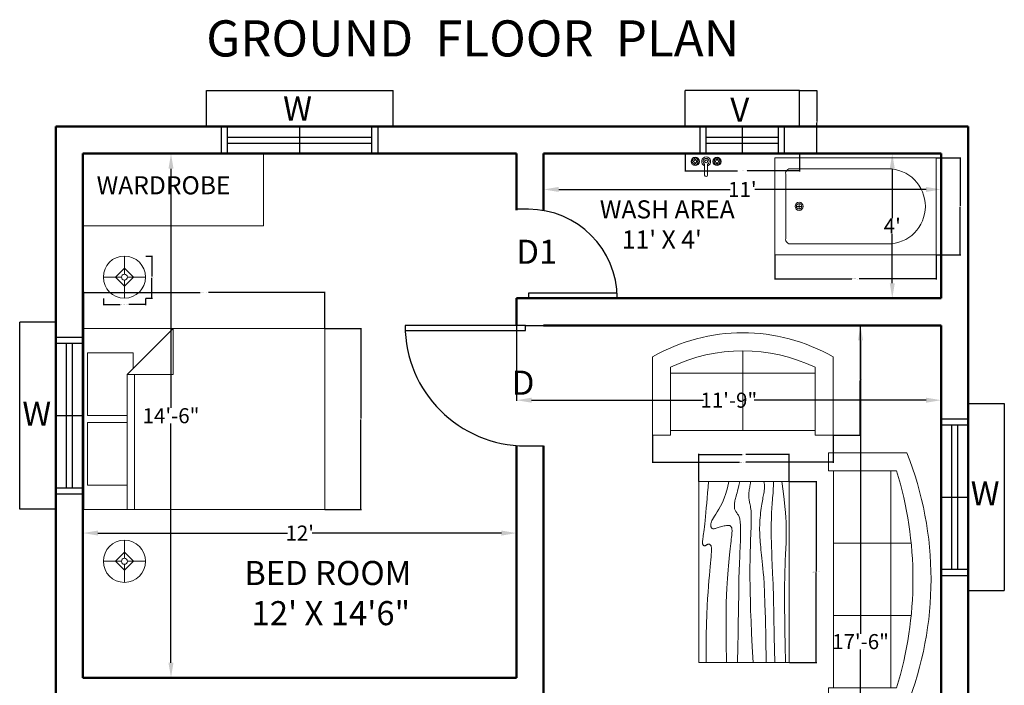
# Model space of a CAD drawing. Units: inches. Extents: x -25 to 789, y -921 to 230.
# Tile 3 of 5: x 5 to 332, y -11 to 209. Entities that reach past the tile are written whole.
import ezdxf

# ---------------------------------------------------------------- set-up
doc = ezdxf.new("R2010")
doc.units = ezdxf.units.IN
doc.header["$MEASUREMENT"] = 0
for name, color, linetype, lineweight in [('A-ANNO-DIMS', 2, 'Continuous', 18), ('A-ANNO-TEXT', 7, 'Continuous', 18), ('A-AREA-IDEN', 3, 'Continuous', 18), ('A-DOOR', 4, 'Continuous', 25), ('A-FLOR-FIXT', 9, 'Continuous', 18), ('A-FURN', 8, 'Continuous', 18), ('A-GLAZ', 4, 'Continuous', 25), ('A-WALL', 7, 'Continuous', 50), ('E-LITE-FIXT', 6, 'Continuous', 18)]:
    doc.layers.add(name, color=color, linetype=linetype, lineweight=lineweight)
doc.styles.get("Standard").update_dxf_attribs({"font": 'arial.ttf'})
doc.dimstyles.get("Standard").update_dxf_attribs({"dimtxt": 0.18, "dimasz": 0.18, "dimexe": 0.18, "dimexo": 0.0625, "dimgap": 0.09, "dimtad": 0, "dimtih": 1, "dimtoh": 1, "dimdec": 1, "dimzin": 0, "dimdsep": 46, "dimlunit": 4, "dimtxsty": 'Standard', "dimcen": 0.09, "dimadec": 0, "dimazin": 0, "dimtfac": 1, "dimtdec": 1, "dimtofl": 0, "dimtmove": 0, "dimatfit": 3, "dimfxl": 1, "dimtolj": 1, "dimtzin": 0, "dimarcsym": 0})

# ---------------------------------------------------------------- blocks, each defined once
blk = doc.blocks.new('*U2')
for p, q in [((0, 0), (0, -6)), ((-40, 0), (-40, -6))]:
    blk.add_line(p, q)
blk.add_lwpolyline([(0, 0), (0, 40), (-1.75, 40), (-1.75, 0)], close=True)
blk.add_arc((0, 0), 40, 90, 180)
blk = doc.blocks.new('*U4')
for p, q in [((-750, 0), (-750, -100)), ((0, 0), (0, -100))]:
    blk.add_line(p, q)
blk.add_lwpolyline([(0, 0), (0, 750), (-43.75, 750), (-43.75, 0)], close=True)
blk.add_arc((0, 0), 750, 90, 180)
blk = doc.blocks.new('Bed - Queen')
for p, q in [((0, -80.00003), (0, 0)), ((0, 0), (59.99999, 0)), ((59.99999, 0), (59.99999, -80.00003)), ((7.99999, -1.2), (28.79998, -1.2)), ((7.99999, -14.4), (7.99999, -1.2)), ((28.79998, -1.2), (28.79998, -14.4)), ((31.19999, -1.2), (51.99999, -1.2)), ((31.19999, -14.4), (31.19999, -1.2)), ((51.99999, -1.2), (51.99999, -16.4)), ((0, -14.4), (44.8, -14.4)), ((59.99999, -29.6), (44.8, -14.4)), ((44.8, -14.4), (44.8, -29.6)), ((44.8, -16.8), (0, -16.8)), ((51.99999, -16.4), (46.79936, -16.4)), ((44.8, -29.6), (59.99999, -29.6)), ((59.99999, -80.00003), (0, -80.00003))]:
    blk.add_line(p, q)
blk = doc.blocks.new('Lamp - Table')
for p, q in [((0, 7), (0, 1)), ((-1, 0), (-7, 0)), ((0, 3), (-3, 0)), ((-3, 0), (0, -3)), ((3, 0), (0, 3)), ((0, -3), (3, 0)), ((1, 0), (7, 0)), ((0, -1), (0, -7))]:
    blk.add_line(p, q)
for radius in [7, 1]:
    blk.add_circle((0, 0), radius)
blk = doc.blocks.new('Faucet - Bathroom top')
for p, q in [((-4.107, 0.125), (-4.375, 0.125)), ((-3.75, 0.4788), (-3.75, 0.75)), ((-3.5, 0.482), (-3.5, 0.75)), ((-3.1461, 0.125), (-2.875, 0.125)), ((3.143, 0.125), (2.875, 0.125)), ((3.5, 0.4788), (3.5, 0.75)), ((3.75, 0.482), (3.75, 0.75)), ((4.1039, 0.125), (4.375, 0.125)), ((-4.1039, -0.125), (-4.375, -0.125)), ((-3.75, -0.4821), (-3.75, -0.75)), ((-3.5, -0.4789), (-3.5, -0.75)), ((-3.143, -0.125), (-2.875, -0.125)), ((-0.5, -0.8639), (-0.5, -4.5)), ((0.5, -4.5), (0.5, -0.8631)), ((3.1461, -0.125), (2.875, -0.125)), ((3.5, -0.4821), (3.5, -0.75)), ((3.75, -0.4789), (3.75, -0.75)), ((4.107, -0.125), (4.375, -0.125))]:
    blk.add_line(p, q)
for centre, radius in [((-3.625, 0), 1.375), ((-4.625, 0), 0.2795), ((-3.625, 0), 0.5), ((-3.625, 1), 0.2795), ((-2.625, 0), 0.2795), ((0, 0), 0.5), ((3.625, 0), 1.375), ((2.625, 0), 0.2795), ((3.625, 0), 0.5), ((3.625, 1), 0.2795), ((4.625, 0), 0.2795), ((-3.625, -1), 0.2795), ((3.625, -1), 0.2795)]:
    blk.add_circle(centre, radius)
for centre, radius, start, end in [((-3.625, 0), 1, 105.2407, 164.2093), ((-3.625, 0), 1, 16.44125, 74.07887), ((0, 0), 1.5, 289.6514, 250.3603), ((0, 0), 1, 300.3431, 239.7554), ((3.625, 0), 1, 106.12, 164.0884), ((3.625, 0), 1, 16.23422, 73.90469), ((-3.625, 0), 1, 196.2342, 253.9047), ((-3.625, 0), 1, 286.12, 344.0884), ((3.625, 0), 1, 196.4413, 254.0789), ((3.625, 0), 1, 285.2407, 344.2093), ((0, -4.5), 0.5, 180, 0)]:
    blk.add_arc(centre, radius, start, end)
blk = doc.blocks.new('Bath Tub - 26 x 60 in.')
for p, q in [((8, -18), (10, -18)), ((9, -17), (9, -19))]:
    blk.add_line(p, q)
blk.add_lwpolyline([(0, -36), (0, 0), (60, 0), (60, -36)], close=True)
for points in [[(4, -30), (4, -6)], [(6, -4), (42, -4)], [(42, -32), (6, -32)]]:
    blk.add_lwpolyline(points)
for radius in [1.5, 1]:
    blk.add_circle((9, -18), radius)
for centre, radius, start, end in [((5.75, -5.75), 1.77, 81.8699, 188.1301), ((42, -18), 14, 270, 90), ((5.75, -30.25), 1.77, 171.8699, 278.1301)]:
    blk.add_arc(centre, radius, start, end)
blk = doc.blocks.new('Sofa - Roundback Loveseat 5 ft.')
for p, q in [((0, -32.44198), (0, -5.99998)), ((-24, -33.99998), (-24, -11.46958)), ((24.00004, -33.99998), (24.00004, -11.46958)), ((-23.9998, -13.38178), (23.99986, -13.38178)), ((-24, -32.44198), (24.00004, -32.44198))]:
    blk.add_line(p, q)
for points in [[(-24, -33.99998), (-30, -33.99998), (-30, -7.99998)], [(30.00004, -7.99998), (30.00004, -33.99998), (24.00004, -33.99998)]]:
    blk.add_lwpolyline(points)
for centre, radius, start, end in [((0, -60.24998), 60.24998, 60.13715, 119.8628), ((0, -61.38438), 55.38444, 64.32083, 115.6792)]:
    blk.add_arc(centre, radius, start, end)
blk = doc.blocks.new('Table - Rectangular Woodgrain 60 x 30 in.')
for p, q in [((0, 0), (0, -30)), ((60, 0), (0, 0)), ((60, -30), (60, 0)), ((0, -30), (60, -30))]:
    blk.add_line(p, q)
for points in [[(0, -2.4), (4.8155, -2.418), (9.0302, -2.4688), (12.709, -2.5477), (15.9167, -2.65), (18.7181, -2.7711), (21.1781, -2.9063), (23.3616, -3.0508), (25.3333, -3.2), (27.1477, -3.3495), (28.8172, -3.4958), (30.3437, -3.636), (31.7291, -3.7667), (32.9756, -3.8849), (34.0849, -3.9875), (35.059, -4.0714), (35.9, -4.1334), (36.6114, -4.1711), (37.2041, -4.1854), (37.6906, -4.1779), (38.0833, -4.15), (38.3948, -4.1034), (38.6375, -4.0396), (38.8239, -3.9602), (38.9666, -3.8667), (39.0764, -3.7608), (39.1573, -3.6448), (39.2116, -3.521), (39.2416, -3.3917), (39.2498, -3.2593), (39.2385, -3.1261), (39.21, -2.9944), (39.1666, -2.8667), (39.111, -2.7447), (39.0468, -2.6281), (38.978, -2.5163), (38.9083, -2.4083), (38.8418, -2.3035), (38.7823, -2.201), (38.7337, -2.1001), (38.7, -2), (38.6844, -1.9003), (38.6875, -1.8021), (38.7094, -1.707), (38.75, -1.6167), (38.8094, -1.5326), (38.8875, -1.4563), (38.9844, -1.3893), (39.1, -1.3333), (39.2351, -1.2896), (39.3937, -1.2583), (39.5804, -1.2396), (39.8, -1.2333), (40.057, -1.2396), (40.3562, -1.2583), (40.7023, -1.2896), (41.1, -1.3333), (41.5547, -1.3895), (42.0755, -1.4573), (42.6721, -1.5361), (43.3542, -1.625), (44.1316, -1.7233), (45.014, -1.8302), (46.0114, -1.9449), (47.1333, -2.0667), (48.3862, -2.1947), (49.7625, -2.3281), (51.2513, -2.4663), (52.8416, -2.6083), (54.5226, -2.7535), (56.2833, -2.9011), (58.1127, -3.0501), (60, -3.2)], [(0, -9.2), (6.5759, -9.0858), (11.9385, -9.0365), (16.2527, -9.0418), (19.6833, -9.0917), (22.3952, -9.1759), (24.5531, -9.2844), (26.322, -9.4069), (27.8666, -9.5333), (29.3241, -9.6553), (30.7203, -9.7719), (32.0532, -9.8837), (33.3208, -9.9917), (34.5213, -10.0965), (35.6526, -10.199), (36.7128, -10.2999), (37.7, -10.4), (38.6129, -10.4996), (39.4531, -10.5969), (40.223, -10.6895), (40.925, -10.775), (41.5613, -10.8512), (42.1344, -10.9156), (42.6465, -10.966), (43.1, -11), (43.4976, -11.0158), (43.8437, -11.0136), (44.143, -10.9942), (44.4, -10.9583), (44.6195, -10.9069), (44.8062, -10.8406), (44.9648, -10.7603), (45.1, -10.6667), (45.2155, -10.5598), (45.3114, -10.4365), (45.3871, -10.2929), (45.4416, -10.125), (45.4743, -9.929), (45.4844, -9.7011), (45.4709, -9.4371), (45.4333, -9.1333), (45.3716, -8.7883), (45.2896, -8.4104), (45.1919, -8.0107), (45.0833, -7.6), (44.9685, -7.1893), (44.8521, -6.7896), (44.7388, -6.4117), (44.6333, -6.0667), (44.54, -5.7628), (44.4614, -5.4979), (44.4001, -5.2675), (44.3583, -5.0667), (44.3384, -4.8909), (44.3427, -4.7354), (44.3736, -4.5956), (44.4333, -4.4667), (44.5236, -4.3453), (44.6427, -4.2333), (44.7884, -4.1339), (44.9583, -4.05), (45.1501, -3.9849), (45.3614, -3.9417), (45.59, -3.9234), (45.8333, -3.9333), (46.0915, -3.9749), (46.3734, -4.0531), (46.6906, -4.1736), (47.0542, -4.3417), (47.4756, -4.5629), (47.9661, -4.8427), (48.5372, -5.1866), (49.2, -5.6), (49.9676, -6.0844), (50.8594, -6.625), (51.8965, -7.2031), (53.1, -7.8), (54.491, -8.3969), (56.0906, -8.975), (57.9199, -9.5156), (60, -10)], [(0, -12.8), (5.1847, -12.9322), (9.6213, -13.0323), (13.3963, -13.1059), (16.5958, -13.1583), (19.3063, -13.1952), (21.614, -13.2219), (23.6054, -13.2439), (25.3666, -13.2667), (26.9728, -13.2947), (28.4531, -13.3281), (29.8256, -13.3663), (31.1083, -13.4083), (32.3191, -13.4535), (33.476, -13.501), (34.597, -13.5501), (35.7, -13.6), (36.7984, -13.6497), (37.8875, -13.6979), (38.9578, -13.743), (40, -13.7833), (41.0047, -13.8174), (41.9625, -13.8438), (42.864, -13.8607), (43.7, -13.8667), (44.4631, -13.8604), (45.1552, -13.8417), (45.7801, -13.8104), (46.3416, -13.7667), (46.8439, -13.7104), (47.2906, -13.6417), (47.6858, -13.5604), (48.0333, -13.4667), (48.3375, -13.3608), (48.6042, -13.2448), (48.8396, -13.121), (49.05, -12.9917), (49.2417, -12.8593), (49.4208, -12.7261), (49.5937, -12.5944), (49.7667, -12.4667), (49.9452, -12.3451), (50.1323, -12.2313), (50.3303, -12.1268), (50.5416, -12.0333), (50.7686, -11.9524), (51.0135, -11.8854), (51.2788, -11.8341), (51.5666, -11.8), (51.8785, -11.7843), (52.2116, -11.7865), (52.562, -11.8059), (52.926, -11.8417), (53.2998, -11.8931), (53.6795, -11.9594), (54.0614, -12.0397), (54.4416, -12.1333), (54.8223, -12.2401), (55.2293, -12.3625), (55.6942, -12.5037), (56.2489, -12.6667), (56.9251, -12.8547), (57.7545, -13.0708), (58.7689, -13.3182), (60, -13.6)], [(0, -18), (5.124, -17.7273), (9.6609, -17.5057), (13.6705, -17.3303), (17.2125, -17.1958), (20.3467, -17.0973), (23.1328, -17.0297), (25.6307, -16.9878), (27.9, -16.9667), (29.9928, -16.9617), (31.9302, -16.9703), (33.7254, -16.9907), (35.3917, -17.0208), (36.9423, -17.0588), (38.3906, -17.1026), (39.7499, -17.1503), (41.0333, -17.2), (42.2519, -17.2496), (43.4073, -17.2969), (44.4986, -17.3395), (45.525, -17.375), (46.4858, -17.4012), (47.3802, -17.4156), (48.2074, -17.416), (48.9667, -17.4), (49.6583, -17.3662), (50.2872, -17.3167), (50.8595, -17.2547), (51.3812, -17.1833), (51.8584, -17.1057), (52.2971, -17.025), (52.7034, -16.9443), (53.0833, -16.8667), (53.443, -16.7951), (53.789, -16.7313), (54.128, -16.6768), (54.4666, -16.6334), (54.8115, -16.6024), (55.1693, -16.5854), (55.5465, -16.5841), (55.95, -16.6), (56.3828, -16.6337), (56.8346, -16.6823), (57.2915, -16.7418), (57.7396, -16.8084), (58.165, -16.878), (58.5539, -16.9469), (58.8924, -17.0111), (59.1666, -17.0667), (59.3679, -17.1107), (59.5078, -17.1438), (59.6032, -17.1675), (59.6708, -17.1833), (59.7275, -17.193), (59.7901, -17.1979), (59.8753, -17.1998), (60, -17.2)], [(0, -22.4), (8.0098, -22.2501), (14.4094, -22.1011), (19.4168, -21.9535), (23.25, -21.8083), (26.1269, -21.6663), (28.2656, -21.5281), (29.884, -21.3947), (31.2, -21.2667), (32.3967, -21.1448), (33.5172, -21.0292), (34.5697, -20.9198), (35.5625, -20.8167), (36.5037, -20.7198), (37.4015, -20.6292), (38.2642, -20.5448), (39.1, -20.4667), (39.9164, -20.3951), (40.7187, -20.3313), (41.5117, -20.2768), (42.3, -20.2333), (43.0883, -20.2024), (43.8812, -20.1854), (44.6836, -20.1841), (45.5, -20.2), (46.3328, -20.234), (47.1747, -20.2844), (48.0163, -20.3488), (48.8479, -20.425), (49.66, -20.5106), (50.4429, -20.6031), (51.1872, -20.7004), (51.8833, -20.8), (52.5246, -20.8999), (53.1166, -20.9995), (53.6681, -21.0983), (54.1875, -21.1958), (54.6834, -21.2919), (55.1646, -21.3859), (55.6394, -21.4777), (56.1167, -21.5667), (56.6028, -21.6515), (57.0961, -21.7266), (57.5929, -21.7852), (58.0896, -21.8208), (58.5823, -21.8268), (59.0674, -21.7964), (59.5412, -21.723), (60, -21.6)], [(0, -25.2), (8.6355, -25.0504), (15.7026, -24.9031), (21.4049, -24.7606), (25.9458, -24.625), (29.529, -24.4988), (32.3578, -24.3844), (34.6359, -24.284), (36.5667, -24.2), (38.3213, -24.1341), (39.9417, -24.0854), (41.437, -24.0523), (42.8167, -24.0333), (44.0901, -24.0268), (45.2667, -24.0313), (46.3557, -24.0451), (47.3667, -24.0667), (48.309, -24.0947), (49.1928, -24.1287), (50.0284, -24.168), (50.826, -24.2125), (51.5959, -24.2617), (52.3483, -24.3151), (53.0935, -24.3725), (53.8417, -24.4334), (54.6009, -24.497), (55.3699, -24.561), (56.1454, -24.6226), (56.9239, -24.6792), (57.7021, -24.7279), (58.4764, -24.7662), (59.2435, -24.7911), (60, -24.8)], [(0, -28.8), (5.6867, -28.6681), (10.45, -28.5698), (14.407, -28.5012), (17.675, -28.4584), (20.3711, -28.4374), (22.6125, -28.4344), (24.5164, -28.4455), (26.2, -28.4667), (27.762, -28.4947), (29.2276, -28.5281), (30.6033, -28.5663), (31.8958, -28.6084), (33.1118, -28.6535), (34.2578, -28.7011), (35.3405, -28.7501), (36.3666, -28.8), (37.3443, -28.8497), (38.288, -28.8974), (39.2137, -28.9412), (40.1375, -28.9792), (41.0753, -29.0093), (42.0432, -29.0297), (43.0572, -29.0384), (44.1333, -29.0333), (45.2936, -29.0114), (46.5843, -28.9641), (48.0579, -28.8816), (49.7666, -28.7542), (51.7629, -28.5721), (54.0989, -28.3255), (56.8272, -28.0048), (60, -27.6)]]:
    blk.add_lwpolyline(points)
blk = doc.blocks.new('Sofa - Roundback 7 ft.')
for p, q in [((-12.00002, -32.4421), (-12.00003, -6.5971)), ((11.99997, -32.4421), (11.99998, -6.5971)), ((-36.000027, -34), (-36.000027, -11.4696)), ((35.99998, -34), (35.99998, -11.4696)), ((-35.999844, -13.3819), (35.9998, -13.3819)), ((-36.000027, -32.4421), (35.99998, -32.4421))]:
    blk.add_line(p, q)
for points in [[(-36.000027, -34), (-42.000027, -34), (-42.000027, -8)], [(41.99998, -8), (41.99998, -34), (35.99998, -34)]]:
    blk.add_lwpolyline(points)
for centre, radius, start, end in [((0, -114.25), 114.25, 68.43141, 111.5686), ((-0.00001, -127.1968), 121.1968, 72.72033, 107.2797)]:
    blk.add_arc(centre, radius, start, end)
blk = doc.blocks.new('*D51')
at = {"layer": 'A-ANNO-DIMS', "color": 0, "lineweight": -2, "transparency": 16777216}
for p, q in [((26.26, -8.92), (26.26, 39.24)), ((170.26, -8.92), (170.26, 39.24))]:
    blk.add_line(p, q, dxfattribs=at)
at = {"layer": 'A-ANNO-DIMS', "color": 0, "lineweight": -3, "transparency": 16777216}
for p, q in [((31.26, 39.06), (94.16, 39.06)), ((165.26, 39.06), (102.36, 39.06))]:
    blk.add_line(p, q, dxfattribs=at)
at = {"layer": 'A-ANNO-DIMS', "color": 0, "transparency": 16777216}
for points in [[(31.26, 39.89), (31.26, 38.23), (26.26, 39.06)], [(165.26, 39.89), (165.26, 38.23), (170.26, 39.06)]]:
    blk.add_solid(points, dxfattribs=at)
at = {"layer": 'Defpoints', "color": 0, "transparency": 16777216}
for p in [(170.26, 39.06), (26.26, -8.98), (170.26, -8.98)]:
    blk.add_point(p, dxfattribs=at)
at = {"layer": 'A-ANNO-DIMS', "color": 0, "transparency": 16777216, "insert": (98.26, 39.06), "char_height": 5, "attachment_point": 5}
blk.add_mtext("\\A1;12'", dxfattribs=at)
blk = doc.blocks.new('*D52')
at = {"layer": 'A-ANNO-DIMS', "color": 0, "lineweight": -2, "transparency": 16777216}
for p, q in [((26.32, 165.02), (55.69, 165.02)), ((55.51, 160.02), (55.51, 80.66)), ((55.51, -3.98), (55.51, 75.38)), ((26.32, -8.98), (55.69, -8.98))]:
    blk.add_line(p, q, dxfattribs=at)
at = {"layer": 'A-ANNO-DIMS', "color": 0, "transparency": 16777216}
for points in [[(54.67, 160.02), (56.34, 160.02), (55.51, 165.02)], [(54.67, -3.98), (56.34, -3.98), (55.51, -8.98)]]:
    blk.add_solid(points, dxfattribs=at)
at = {"layer": 'Defpoints', "color": 0, "transparency": 16777216}
for p in [(26.26, 165.02), (55.51, 165.02), (26.26, -8.98)]:
    blk.add_point(p, dxfattribs=at)
at = {"layer": 'A-ANNO-DIMS', "color": 0, "transparency": 16777216, "insert": (55.51, 78.02), "char_height": 5, "attachment_point": 5}
blk.add_mtext('\\A1;14\'-6"', dxfattribs=at)
blk = doc.blocks.new('*D53')
at = {"layer": 'A-ANNO-DIMS', "color": 0, "lineweight": -2, "transparency": 16777216}
for p, q in [((311.2, 165.02), (294.87, 165.02)), ((295.05, 160.02), (295.05, 143.61)), ((295.05, 122.02), (295.05, 138.43)), ((311.2, 117.02), (294.87, 117.02))]:
    blk.add_line(p, q, dxfattribs=at)
at = {"layer": 'A-ANNO-DIMS', "color": 0, "transparency": 16777216}
for points in [[(294.22, 160.02), (295.89, 160.02), (295.05, 165.02)], [(294.22, 122.02), (295.89, 122.02), (295.05, 117.02)]]:
    blk.add_solid(points, dxfattribs=at)
at = {"layer": 'Defpoints', "color": 0, "transparency": 16777216}
for p in [(311.26, 165.02), (295.05, 117.02), (311.26, 117.02)]:
    blk.add_point(p, dxfattribs=at)
at = {"layer": 'A-ANNO-DIMS', "color": 0, "transparency": 16777216, "insert": (295.05, 141.02), "char_height": 5, "attachment_point": 5}
blk.add_mtext("\\A1;4'", dxfattribs=at)
blk = doc.blocks.new('*D54')
at = {"layer": 'A-ANNO-DIMS', "color": 0, "lineweight": -2, "transparency": 16777216}
for p, q in [((179.26, 164.96), (179.26, 152.95)), ((311.26, 164.96), (311.26, 152.95)), ((184.26, 153.13), (241.16, 153.13)), ((306.26, 153.13), (249.36, 153.13))]:
    blk.add_line(p, q, dxfattribs=at)
at = {"layer": 'A-ANNO-DIMS', "color": 0, "transparency": 16777216}
for points in [[(184.26, 153.97), (184.26, 152.3), (179.26, 153.13)], [(306.26, 153.97), (306.26, 152.3), (311.26, 153.13)]]:
    blk.add_solid(points, dxfattribs=at)
at = {"layer": 'Defpoints', "color": 0, "transparency": 16777216}
for p in [(179.26, 165.02), (311.26, 165.02), (311.26, 153.13)]:
    blk.add_point(p, dxfattribs=at)
at = {"layer": 'A-ANNO-DIMS', "color": 0, "transparency": 16777216, "insert": (245.26, 153.13), "char_height": 5, "attachment_point": 5}
blk.add_mtext("\\A1;11'", dxfattribs=at)
blk = doc.blocks.new('*D55')
at = {"layer": 'A-ANNO-DIMS', "color": 0, "lineweight": -2, "transparency": 16777216}
for p, q in [((170.26, 107.96), (170.26, 82.99)), ((311.26, 107.96), (311.26, 82.99)), ((175.26, 83.17), (232.32, 83.17)), ((306.26, 83.17), (249.2, 83.17))]:
    blk.add_line(p, q, dxfattribs=at)
at = {"layer": 'A-ANNO-DIMS', "color": 0, "transparency": 16777216}
for points in [[(175.26, 84), (175.26, 82.33), (170.26, 83.17)], [(306.26, 84), (306.26, 82.33), (311.26, 83.17)]]:
    blk.add_solid(points, dxfattribs=at)
at = {"layer": 'Defpoints', "color": 0, "transparency": 16777216}
for p in [(170.26, 108.02), (311.26, 108.02), (311.26, 83.17)]:
    blk.add_point(p, dxfattribs=at)
at = {"layer": 'A-ANNO-DIMS', "color": 0, "transparency": 16777216, "insert": (240.76, 83.17), "char_height": 5, "attachment_point": 5}
blk.add_mtext('\\A1;11\'-9"', dxfattribs=at)
blk = doc.blocks.new('*D56')
at = {"layer": 'A-ANNO-DIMS', "color": 0, "lineweight": -2, "transparency": 16777216}
for p, q in [((311.2, 108.02), (284.32, 108.02)), ((284.5, 103.02), (284.5, 5.66)), ((284.5, -96.98), (284.5, 0.38)), ((311.2, -101.98), (284.32, -101.98))]:
    blk.add_line(p, q, dxfattribs=at)
at = {"layer": 'A-ANNO-DIMS', "color": 0, "transparency": 16777216}
for points in [[(283.67, 103.02), (285.33, 103.02), (284.5, 108.02)], [(283.67, -96.98), (285.33, -96.98), (284.5, -101.98)]]:
    blk.add_solid(points, dxfattribs=at)
at = {"layer": 'Defpoints', "color": 0, "transparency": 16777216}
for p in [(284.5, 108.02), (311.26, 108.02), (311.26, -101.98)]:
    blk.add_point(p, dxfattribs=at)
at = {"layer": 'A-ANNO-DIMS', "color": 0, "transparency": 16777216, "insert": (284.5, 3.02), "char_height": 5, "attachment_point": 5}
blk.add_mtext('\\A1;17\'-6"', dxfattribs=at)
blk = doc.blocks.new('WIN-W-SUNSHADE')
at = {"ltscale": 2}
for p, q in [((0, 9), (0, 21)), ((0, 21), (62, 21)), ((62, 9), (62, 21)), ((5, 9), (0, 9)), ((57, 9), (62, 9))]:
    blk.add_line(p, q, dxfattribs=at)
for p, q in [((5, 0), (5, 9)), ((57, 0), (57, 9))]:
    blk.add_line(p, q)
blk = doc.blocks.new('WIN-V-SUNSHADE')
for p, q in [((0, 9), (0, 21)), ((38, 21), (0, 21)), ((38, 9), (38, 21)), ((5, 9), (0, 9)), ((5, 0), (5, 9)), ((33, 0), (33, 9)), ((33, 9), (38, 9))]:
    blk.add_line(p, q)
blk = doc.blocks.new('*D83')
at = {"layer": 'A-ANNO-DIMS', "color": 0, "lineweight": -2, "transparency": 16777216}
for p, q in [((226.26, 164.96), (226.26, 159.14)), ((264.26, 164.96), (264.26, 159.14)), ((226.44, 159.32), (243.67, 159.32)), ((264.08, 159.32), (246.85, 159.32))]:
    blk.add_line(p, q, dxfattribs=at)
at = {"layer": 'A-ANNO-DIMS', "color": 0, "transparency": 16777216}
for points in [[(226.44, 159.35), (226.44, 159.29), (226.26, 159.32)], [(264.08, 159.35), (264.08, 159.29), (264.26, 159.32)]]:
    blk.add_solid(points, dxfattribs=at)
at = {"layer": 'Defpoints', "color": 0, "transparency": 16777216}
for p in [(226.26, 165.02), (264.26, 165.02), (264.26, 159.32)]:
    blk.add_point(p, dxfattribs=at)
at = {"layer": 'A-ANNO-DIMS', "color": 0, "transparency": 16777216, "insert": (245.26, 159.32), "char_height": 0.18, "attachment_point": 5}
blk.add_mtext('\\A1;VENTILATOR V 3\'-2" TYP.', dxfattribs=at)
blk = doc.blocks.new('*D84')
at = {"layer": 'A-ANNO-DIMS', "color": 0, "lineweight": -2, "transparency": 16777216}
for p, q in [((264.32, 186.02), (270.14, 186.02)), ((269.96, 185.84), (269.96, 175.7)), ((269.96, 165.2), (269.96, 175.34)), ((264.32, 165.02), (270.14, 165.02))]:
    blk.add_line(p, q, dxfattribs=at)
at = {"layer": 'A-ANNO-DIMS', "color": 0, "transparency": 16777216}
for points in [[(269.93, 185.84), (269.99, 185.84), (269.96, 186.02)], [(269.93, 165.2), (269.99, 165.2), (269.96, 165.02)]]:
    blk.add_solid(points, dxfattribs=at)
at = {"layer": 'Defpoints', "color": 0, "transparency": 16777216}
for p in [(264.26, 186.02), (269.96, 186.02), (264.26, 165.02)]:
    blk.add_point(p, dxfattribs=at)
at = {"layer": 'A-ANNO-DIMS', "color": 0, "transparency": 16777216, "insert": (269.96, 175.52), "char_height": 0.18, "attachment_point": 5}
blk.add_mtext('\\A1;1\'-9" TYP.', dxfattribs=at)
blk = doc.blocks.new('*D85')
at = {"layer": 'A-ANNO-DIMS', "color": 0, "lineweight": -2, "transparency": 16777216}
for p, q in [((26.58, 106.99), (26.58, 119.11)), ((26.76, 118.93), (65.17, 118.93)), ((106.4, 118.93), (68, 118.93)), ((106.58, 106.99), (106.58, 119.11))]:
    blk.add_line(p, q, dxfattribs=at)
at = {"layer": 'A-ANNO-DIMS', "color": 0, "transparency": 16777216}
for points in [[(26.76, 118.96), (26.76, 118.9), (26.58, 118.93)], [(106.4, 118.96), (106.4, 118.9), (106.58, 118.93)]]:
    blk.add_solid(points, dxfattribs=at)
at = {"layer": 'Defpoints', "color": 0, "transparency": 16777216}
for p in [(26.58, 118.93), (26.58, 106.93), (106.58, 106.93)]:
    blk.add_point(p, dxfattribs=at)
at = {"layer": 'A-ANNO-DIMS', "color": 0, "transparency": 16777216, "insert": (66.58, 118.93), "char_height": 0.18, "attachment_point": 5}
blk.add_mtext('\\A1;QUEEN BED 6\'-8" TYP.', dxfattribs=at)
blk = doc.blocks.new('*D86')
at = {"layer": 'A-ANNO-DIMS', "color": 0, "lineweight": -2, "transparency": 16777216}
for p, q in [((106.65, 106.93), (118.76, 106.93)), ((118.58, 106.75), (118.58, 77.11)), ((118.58, 47.11), (118.58, 76.74)), ((106.65, 46.93), (118.76, 46.93))]:
    blk.add_line(p, q, dxfattribs=at)
at = {"layer": 'A-ANNO-DIMS', "color": 0, "transparency": 16777216}
for points in [[(118.55, 106.75), (118.61, 106.75), (118.58, 106.93)], [(118.55, 47.11), (118.61, 47.11), (118.58, 46.93)]]:
    blk.add_solid(points, dxfattribs=at)
at = {"layer": 'Defpoints', "color": 0, "transparency": 16777216}
for p in [(106.58, 106.93), (118.58, 106.93), (106.58, 46.93)]:
    blk.add_point(p, dxfattribs=at)
at = {"layer": 'A-ANNO-DIMS', "color": 0, "transparency": 16777216, "insert": (118.58, 76.93), "char_height": 0.18, "attachment_point": 5}
blk.add_mtext('\\A1;5\'-0" TYP.', dxfattribs=at)
blk = doc.blocks.new('*D89')
at = {"layer": 'A-ANNO-DIMS', "color": 0, "lineweight": -2, "transparency": 16777216}
for p, q in [((33.05, 116.96), (33.05, 114.74)), ((33.23, 114.92), (38.6, 114.92)), ((46.87, 114.92), (41.51, 114.92)), ((47.05, 116.96), (47.05, 114.74))]:
    blk.add_line(p, q, dxfattribs=at)
at = {"layer": 'A-ANNO-DIMS', "color": 0, "transparency": 16777216}
for points in [[(33.23, 114.95), (33.23, 114.89), (33.05, 114.92)], [(46.87, 114.95), (46.87, 114.89), (47.05, 114.92)]]:
    blk.add_solid(points, dxfattribs=at)
at = {"layer": 'Defpoints', "color": 0, "transparency": 16777216}
for p in [(33.05, 117.02), (47.05, 117.02), (47.05, 114.92)]:
    blk.add_point(p, dxfattribs=at)
at = {"layer": 'A-ANNO-DIMS', "color": 0, "transparency": 16777216, "insert": (40.05, 114.92), "char_height": 0.18, "attachment_point": 5}
blk.add_mtext('\\A1;TABLE LAMP 1\'-2" TYP.', dxfattribs=at)
blk = doc.blocks.new('*D90')
at = {"layer": 'A-ANNO-DIMS', "color": 0, "lineweight": -2, "transparency": 16777216}
for p, q in [((47.12, 131.02), (49.33, 131.02)), ((49.15, 130.84), (49.15, 124.2)), ((49.15, 117.2), (49.15, 123.84)), ((47.12, 117.02), (49.33, 117.02))]:
    blk.add_line(p, q, dxfattribs=at)
at = {"layer": 'A-ANNO-DIMS', "color": 0, "transparency": 16777216}
for points in [[(49.12, 130.84), (49.18, 130.84), (49.15, 131.02)], [(49.12, 117.2), (49.18, 117.2), (49.15, 117.02)]]:
    blk.add_solid(points, dxfattribs=at)
at = {"layer": 'Defpoints', "color": 0, "transparency": 16777216}
for p in [(47.05, 131.02), (49.15, 131.02), (47.05, 117.02)]:
    blk.add_point(p, dxfattribs=at)
at = {"layer": 'A-ANNO-DIMS', "color": 0, "transparency": 16777216, "insert": (49.15, 124.02), "char_height": 0.18, "attachment_point": 5}
blk.add_mtext('\\A1;1\'-2" TYP.', dxfattribs=at)
blk = doc.blocks.new('*D91')
at = {"layer": 'A-ANNO-DIMS', "color": 0, "lineweight": -2, "transparency": 16777216}
for p, q in [((260.89, 56.13), (270, 56.13)), ((269.82, 55.95), (269.82, 26.31)), ((269.82, -3.69), (269.82, 25.95)), ((260.89, -3.87), (270, -3.87))]:
    blk.add_line(p, q, dxfattribs=at)
at = {"layer": 'A-ANNO-DIMS', "color": 0, "transparency": 16777216}
for points in [[(269.79, 55.95), (269.85, 55.95), (269.82, 56.13)], [(269.79, -3.69), (269.85, -3.69), (269.82, -3.87)]]:
    blk.add_solid(points, dxfattribs=at)
at = {"layer": 'Defpoints', "color": 0, "transparency": 16777216}
for p in [(260.82, 56.13), (269.82, 56.13), (260.82, -3.87)]:
    blk.add_point(p, dxfattribs=at)
at = {"layer": 'A-ANNO-DIMS', "color": 0, "transparency": 16777216, "insert": (269.82, 26.13), "char_height": 0.18, "attachment_point": 5}
blk.add_mtext('\\A1;TABLE 60X30 5\'-0" TYP.', dxfattribs=at)
blk = doc.blocks.new('*D92')
at = {"layer": 'A-ANNO-DIMS', "color": 0, "lineweight": -2, "transparency": 16777216}
for p, q in [((230.82, 56.19), (230.82, 65.31)), ((231, 65.13), (245.18, 65.13)), ((260.64, 65.13), (246.46, 65.13)), ((260.82, 56.19), (260.82, 65.31))]:
    blk.add_line(p, q, dxfattribs=at)
at = {"layer": 'A-ANNO-DIMS', "color": 0, "transparency": 16777216}
for points in [[(231, 65.16), (231, 65.1), (230.82, 65.13)], [(260.64, 65.16), (260.64, 65.1), (260.82, 65.13)]]:
    blk.add_solid(points, dxfattribs=at)
at = {"layer": 'Defpoints', "color": 0, "transparency": 16777216}
for p in [(230.82, 65.13), (230.82, 56.13), (260.82, 56.13)]:
    blk.add_point(p, dxfattribs=at)
at = {"layer": 'A-ANNO-DIMS', "color": 0, "transparency": 16777216, "insert": (245.82, 65.13), "char_height": 0.18, "attachment_point": 5}
blk.add_mtext('\\A1;2\'-6" TYP.', dxfattribs=at)
blk = doc.blocks.new('*D97')
at = {"layer": 'A-ANNO-DIMS', "color": 0, "lineweight": -2, "transparency": 16777216}
for p, q in [((256.09, 131.41), (256.09, 123.27)), ((309.61, 131.41), (309.61, 123.27)), ((256.27, 123.45), (281.66, 123.45)), ((309.43, 123.45), (284.04, 123.45))]:
    blk.add_line(p, q, dxfattribs=at)
at = {"layer": 'A-ANNO-DIMS', "color": 0, "transparency": 16777216}
for points in [[(256.27, 123.48), (256.27, 123.42), (256.09, 123.45)], [(309.43, 123.48), (309.43, 123.42), (309.61, 123.45)]]:
    blk.add_solid(points, dxfattribs=at)
at = {"layer": 'Defpoints', "color": 0, "transparency": 16777216}
for p in [(256.09, 131.47), (309.61, 131.47), (309.61, 123.45)]:
    blk.add_point(p, dxfattribs=at)
at = {"layer": 'A-ANNO-DIMS', "color": 0, "transparency": 16777216, "insert": (282.85, 123.45), "char_height": 0.18, "attachment_point": 5}
blk.add_mtext('\\A1;BATH TUB 4\'-5 1/2"', dxfattribs=at)
blk = doc.blocks.new('*D98')
at = {"layer": 'A-ANNO-DIMS', "color": 0, "lineweight": -2, "transparency": 16777216}
for p, q in [((309.67, 163.58), (317.82, 163.58)), ((317.64, 163.4), (317.64, 147.71)), ((317.64, 131.65), (317.64, 147.35)), ((309.67, 131.47), (317.82, 131.47))]:
    blk.add_line(p, q, dxfattribs=at)
at = {"layer": 'A-ANNO-DIMS', "color": 0, "transparency": 16777216}
for points in [[(317.61, 163.4), (317.67, 163.4), (317.64, 163.58)], [(317.61, 131.65), (317.67, 131.65), (317.64, 131.47)]]:
    blk.add_solid(points, dxfattribs=at)
at = {"layer": 'Defpoints', "color": 0, "transparency": 16777216}
for p in [(309.61, 163.58), (317.64, 163.58), (309.61, 131.47)]:
    blk.add_point(p, dxfattribs=at)
at = {"layer": 'A-ANNO-DIMS', "color": 0, "transparency": 16777216, "insert": (317.64, 147.53), "char_height": 0.18, "attachment_point": 5}
blk.add_mtext('\\A1;2\'-8"', dxfattribs=at)
blk = doc.blocks.new('*D99')
at = {"layer": 'A-ANNO-DIMS', "color": 0, "lineweight": -2, "transparency": 16777216}
for p, q in [((215.39, 71.49), (215.39, 62.37)), ((275.39, 71.49), (275.39, 62.37)), ((215.57, 62.55), (244.36, 62.55)), ((275.21, 62.55), (246.41, 62.55))]:
    blk.add_line(p, q, dxfattribs=at)
at = {"layer": 'A-ANNO-DIMS', "color": 0, "transparency": 16777216}
for points in [[(215.57, 62.58), (215.57, 62.52), (215.39, 62.55)], [(275.21, 62.58), (275.21, 62.52), (275.39, 62.55)]]:
    blk.add_solid(points, dxfattribs=at)
at = {"layer": 'Defpoints', "color": 0, "transparency": 16777216}
for p in [(215.39, 71.55), (275.39, 71.55), (275.39, 62.55)]:
    blk.add_point(p, dxfattribs=at)
at = {"layer": 'A-ANNO-DIMS', "color": 0, "transparency": 16777216, "insert": (245.39, 62.55), "char_height": 0.18, "attachment_point": 5}
blk.add_mtext('\\A1;LOVESEAT 5\'-0"', dxfattribs=at)
blk = doc.blocks.new('*D100')
at = {"layer": 'A-ANNO-DIMS', "color": 0, "lineweight": -2, "transparency": 16777216}
for p, q in [((275.45, 108.22), (284.57, 108.22)), ((284.39, 108.04), (284.39, 90.07)), ((284.39, 71.73), (284.39, 89.7)), ((275.45, 71.55), (284.57, 71.55))]:
    blk.add_line(p, q, dxfattribs=at)
at = {"layer": 'A-ANNO-DIMS', "color": 0, "transparency": 16777216}
for points in [[(284.36, 108.04), (284.42, 108.04), (284.39, 108.22)], [(284.36, 71.73), (284.42, 71.73), (284.39, 71.55)]]:
    blk.add_solid(points, dxfattribs=at)
at = {"layer": 'Defpoints', "color": 0, "transparency": 16777216}
for p in [(275.39, 108.22), (284.39, 108.22), (275.39, 71.55)]:
    blk.add_point(p, dxfattribs=at)
at = {"layer": 'A-ANNO-DIMS', "color": 0, "transparency": 16777216, "insert": (284.39, 89.88), "char_height": 0.18, "attachment_point": 5}
blk.add_mtext('\\A1;3\'-0 1/2"', dxfattribs=at)

msp = doc.modelspace()

# ---------------------------------------------------------------- linework, layer by layer
at = {"layer": 'A-FURN'}
for p, q in [((26.26, 165.02), (26.26, 141.02)), ((86.26, 141.02), (86.26, 165.02)), ((26.26, 141.02), (86.26, 141.02))]:
    msp.add_line(p, q, dxfattribs=at)
at = {"layer": 'A-GLAZ'}
for p, q in [((74.26, 165.02), (74.26, 174.02)), ((98.26, 165.02), (98.26, 174.02)), ((122.26, 165.02), (122.26, 174.02)), ((233.26, 165.02), (233.26, 174.02)), ((245.26, 165.02), (245.26, 174.02)), ((257.26, 165.02), (257.26, 174.02)), ((74.26, 170.52), (122.26, 170.52)), ((233.26, 170.52), (257.26, 170.52)), ((74.26, 168.52), (122.26, 168.52)), ((233.26, 168.52), (257.26, 168.52)), ((26.26, 102.02), (17.26, 102.02)), ((20.76, 54.02), (20.76, 102.02)), ((22.76, 54.02), (22.76, 102.02)), ((26.26, 78.02), (17.26, 78.02)), ((311.26, 75.02), (320.26, 75.02)), ((314.76, 75.02), (314.76, 27.02)), ((316.76, 75.02), (316.76, 27.02)), ((26.26, 54.02), (17.26, 54.02)), ((311.26, 51.02), (320.26, 51.02)), ((311.26, 27.02), (320.26, 27.02))]:
    msp.add_line(p, q, dxfattribs=at)
at = {"layer": 'A-WALL'}
for p, q in [((17.26, 174.02), (179.26, 174.02)), ((17.26, -17.98), (17.26, 174.02)), ((179.26, 174.02), (320.26, 174.02)), ((320.26, 174.02), (320.26, 108.02)), ((26.26, -8.98), (26.26, 165.02)), ((26.26, 165.02), (170.26, 165.02)), ((170.26, 146.29), (170.26, 165.02)), ((179.26, 165.02), (311.26, 165.02)), ((179.26, 146.11), (179.26, 165.02)), ((311.26, 165.02), (311.26, 117.02)), ((311.26, 117.02), (170.26, 117.02)), ((170.26, 108.02), (170.26, 117.02)), ((311.26, 108.02), (179.26, 108.02)), ((311.26, 108.02), (311.26, -101.98)), ((320.26, 108.02), (320.26, -314.98)), ((170.26, -8.98), (170.26, 68.13)), ((179.26, -17.98), (179.26, 68.02)), ((26.26, -8.98), (170.26, -8.98))]:
    msp.add_line(p, q, dxfattribs=at)

# ---------------------------------------------------------------- block references
at = {"layer": 'A-DOOR', "xscale": 0.0393700787401575, "yscale": 0.0393700787401575, "zscale": 0.0393700787401575, "rotation": 270}
msp.add_blockref('*U4', (174.2, 117.02), dxfattribs=at)
at = {"layer": 'A-DOOR', "rotation": 90}
msp.add_blockref('*U2', (173.26, 108.02), dxfattribs=at)
at = {"layer": 'A-FLOR-FIXT'}
msp.add_blockref('Faucet - Bathroom top', (233.23, 162.42), dxfattribs=at)
at = {"layer": 'A-FLOR-FIXT', "xscale": 0.8919294306306255, "yscale": 0.8919294306306255, "zscale": 0.8919294306306255}
msp.add_blockref('Bath Tub - 26 x 60 in.', (256.09, 163.58), dxfattribs=at)
at = {"layer": 'A-FURN'}
msp.add_blockref('Sofa - Roundback Loveseat 5 ft.', (245.39, 105.55), dxfattribs=at)
for name, p, rotation in [('Bed - Queen', (26.58, 46.93), 90), ('Sofa - Roundback 7 ft.', (307.92, 23.71), 270), ('Table - Rectangular Woodgrain 60 x 30 in.', (230.82, -3.87), 90)]:
    msp.add_blockref(name, p, dxfattribs=dict(at, rotation=rotation))
at = {"layer": 'A-GLAZ'}
for name, p in [('WIN-W-SUNSHADE', (67.26, 165.02)), ('WIN-V-SUNSHADE', (226.26, 165.02))]:
    msp.add_blockref(name, p, dxfattribs=at)
for p, rotation in [((26.26, 47.02), 90.00000000000021), ((311.26, 82.02), 270.0000000000001)]:
    msp.add_blockref('WIN-W-SUNSHADE', p, dxfattribs=dict(at, rotation=rotation))
at = {"layer": 'E-LITE-FIXT'}
for p in [(40.05, 124.02), (40.05, 29.69)]:
    msp.add_blockref('Lamp - Table', p, dxfattribs=at)

# ---------------------------------------------------------------- texts
at = {"layer": 'A-ANNO-TEXT'}
for s, p in [('W', (92.74, 176.01)), ('V', (241.26, 175.58)), ('D1', (170.21, 128.44)), ('D', (168.7, 84.97)), ('W', (6.13, 74.72)), ('W', (321.09, 48.22))]:
    msp.add_text(s, height=8, dxfattribs=at).set_placement(p)
at = {"layer": 'A-ANNO-TEXT', "insert": (67.21, 209.27), "char_height": 12, "attachment_point": 1}
msp.add_mtext_dynamic_manual_height_columns('GROUND  FLOOR  PLAN', width=235.2118, gutter_width=1, heights=[0], dxfattribs=at)
at = {"layer": 'A-AREA-IDEN', "attachment_point": 1}
for s, insert, char_height in [('WARDROBE', (30.81, 157.51), 6), ("WASH AREA\\P    11' X 4'", (197.92, 149.52), 6), ('BED ROOM\\P 12\' X 14\'6"', (79.82, 29.81), 8)]:
    msp.add_mtext_dynamic_manual_height_columns(s, width=99.8363, gutter_width=1, heights=[0], dxfattribs=dict(at, insert=insert, char_height=char_height))

# ---------------------------------------------------------------- dimensions: what is measured, and where the dimension line sits
at = {"layer": 'A-ANNO-DIMS'}
for base, p1, p2, angle, text, picture, middle in [((269.96, 186.02), (264.26, 165.02), (264.26, 186.02), 90, '<> TYP.', '*D84', (269.96, 175.52)), ((49.15, 131.02), (47.05, 117.02), (47.05, 131.02), 90, '<> TYP.', '*D90', (49.15, 124.02)), ((26.58, 118.93), (106.58, 106.93), (26.58, 106.93), 180, 'QUEEN BED <> TYP.', '*D85', (66.58, 118.93)), ((118.58, 106.93), (106.58, 46.93), (106.58, 106.93), 90, '<> TYP.', '*D86', (118.58, 76.93)), ((230.82, 65.13), (260.82, 56.13), (230.82, 56.13), 180, '<> TYP.', '*D92', (245.82, 65.13)), ((269.82, 56.13), (260.82, -3.87), (260.82, 56.13), 90, 'TABLE 60X30 <> TYP.', '*D91', (269.82, 26.13))]:
    dim = msp.add_linear_dim(base=base, p1=p1, p2=p2, angle=angle, text=text, dimstyle='Standard', override={"dimdec": 1, "dimrnd": 0, "dimzin": 1, "dimlunit": 4, "dimfrac": 2}, dxfattribs=at)
    dim.commit()
    dim.dimension.update_dxf_attribs({"geometry": picture, "text_midpoint": middle})
for base, p1, p2, override, picture, middle in [((55.51, 165.02), (26.26, -8.98), (26.26, 165.02), {"dimtxt": 5, "dimasz": 5, "dimclrd": 0, "dimclre": 0, "dimclrt": 0}, '*D52', (55.51, 78.02)), ((295.05, 117.02), (311.26, 165.02), (311.26, 117.02), {"dimtxt": 5, "dimasz": 5, "dimclrd": 0, "dimclre": 0, "dimclrt": 0}, '*D53', (295.05, 141.02)), ((317.64, 163.58), (309.61, 131.47), (309.61, 163.58), {"dimdec": 1, "dimrnd": 0, "dimzin": 1, "dimlunit": 4, "dimfrac": 2}, '*D98', (317.64, 147.53)), ((284.5, 108.02), (311.26, -101.98), (311.26, 108.02), {"dimtxt": 5, "dimasz": 5, "dimclrd": 0, "dimclre": 0, "dimclrt": 0}, '*D56', (284.5, 3.02)), ((284.39, 108.22), (275.39, 71.55), (275.39, 108.22), {"dimdec": 1, "dimrnd": 0, "dimzin": 1, "dimlunit": 4, "dimfrac": 2}, '*D100', (284.39, 89.88))]:
    dim = msp.add_linear_dim(base=base, p1=p1, p2=p2, angle=90, dimstyle='Standard', override=override, dxfattribs=at)
    dim.commit()
    dim.dimension.update_dxf_attribs({"geometry": picture, "text_midpoint": middle})
for base, p1, p2, override, picture, middle in [((311.26, 153.13), (179.26, 165.02), (311.26, 165.02), {"dimtxt": 5, "dimasz": 5, "dimclrd": 0, "dimclre": 0, "dimclrt": 0}, '*D54', (245.26, 153.13)), ((311.26, 83.17), (170.26, 108.02), (311.26, 108.02), {"dimtxt": 5, "dimasz": 5, "dimclrd": 0, "dimclre": 0, "dimclrt": 0}, '*D55', (240.76, 83.17)), ((170.26, 39.06), (26.26, -8.98), (170.26, -8.98), {"dimtxt": 5, "dimasz": 5, "dimclrd": 0, "dimclre": 0, "dimclrt": 0, "dimlwd": -3}, '*D51', (98.26, 39.06))]:
    dim = msp.add_linear_dim(base=base, p1=p1, p2=p2, dimstyle='Standard', override=override, dxfattribs=at)
    dim.commit()
    dim.dimension.update_dxf_attribs({"geometry": picture, "text_midpoint": middle})
for base, p1, p2, text, picture, middle in [((264.26, 159.32), (226.26, 165.02), (264.26, 165.02), 'VENTILATOR V <> TYP.', '*D83', (245.26, 159.32)), ((309.61, 123.45), (256.09, 131.47), (309.61, 131.47), 'BATH TUB <>', '*D97', (282.85, 123.45)), ((47.05, 114.92), (33.05, 117.02), (47.05, 117.02), 'TABLE LAMP <> TYP.', '*D89', (40.05, 114.92)), ((275.39, 62.55), (215.39, 71.55), (275.39, 71.55), 'LOVESEAT <>', '*D99', (245.39, 62.55))]:
    dim = msp.add_linear_dim(base=base, p1=p1, p2=p2, text=text, dimstyle='Standard', override={"dimdec": 1, "dimrnd": 0, "dimzin": 1, "dimlunit": 4, "dimfrac": 2}, dxfattribs=at)
    dim.commit()
    dim.dimension.update_dxf_attribs({"geometry": picture, "text_midpoint": middle})

doc.saveas('drawing.dxf')
